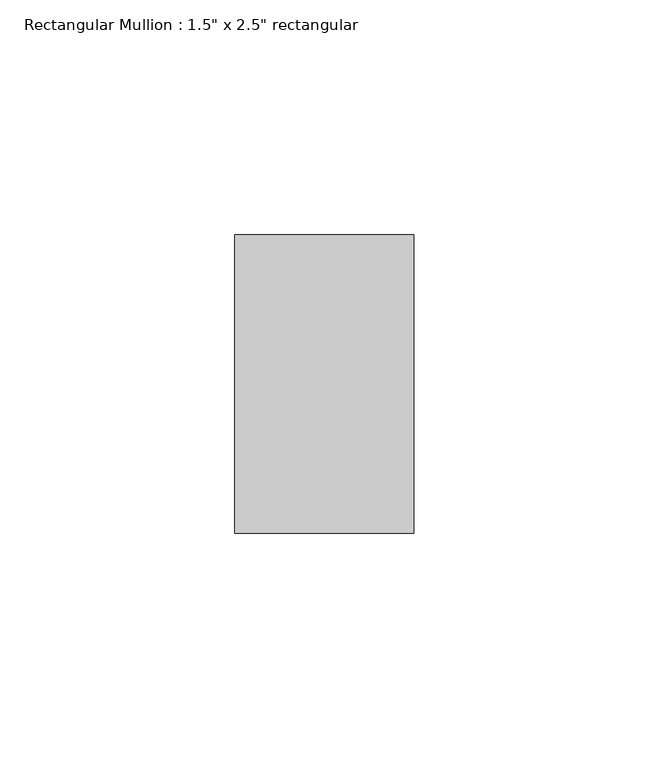
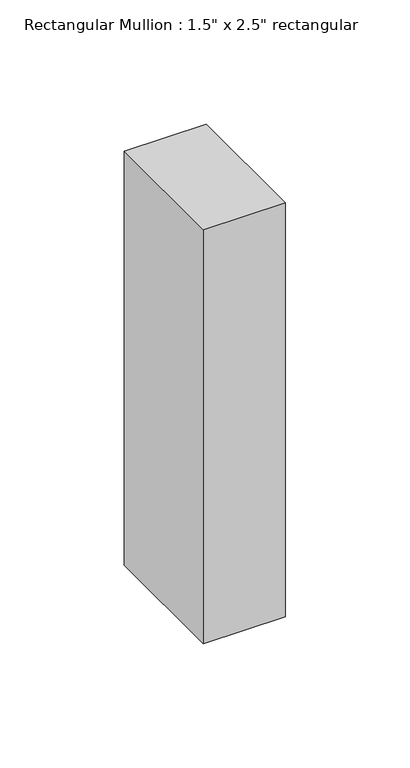
"""IFC4 building model written with IfcOpenShell, lengths in millimetres: member geometry."""

from ifc_helpers import new_model, si_unit, frame, origin, place, context, project, spatial, polyline, outline, extrude, source, transform, mapped, element, save


def member_ff422208(model_context):
    return source(origin(), model_context, "Body", "SweptSolid", [
        extrude(outline(polyline([(0.0, 31.75), (0.0, -31.75), (-38.1, -31.75), (-38.1, 31.75), (0.0, 31.75)])), frame((0.0, 0.0, -203.2), z_axis=(0.0, 0.0, 1.0), x_axis=(1.0, 0.0, 0.0)), (0.0, 0.0, 1.0), 203.2),
    ])


if __name__ == "__main__":
    model = new_model("IFC4")
    model_context = context("Model", 3, world=origin())
    ifc_project = project(units=[si_unit("LENGTHUNIT", "METRE", prefix="MILLI")], contexts=[model_context])
    site = spatial("IfcSite", under=ifc_project)
    building = spatial("IfcBuilding", under=site)
    placement = place(None, origin())
    member_shape = member_ff422208(model_context)
    element("IfcMember", 1, ObjectType="Rectangular Mullion : 1.5\" x 2.5\" rectangular", at=placement, inside=building, context=model_context, shape_type="MappedRepresentation", body=[
        mapped(member_shape, transform((0.0, 0.0, 0.0), x_axis=(1.0, 0.0, 0.0), y_axis=(0.0, 1.0, 0.0), z_axis=(0.0, 0.0, 1.0))),
    ])
    save(model, "model.ifc")

# Revit data of these elements
# Type "Rectangular Mullion : 1.5\" x 2.5\" rectangular"
#   built-in parameter 1007304 = 0.208333 (stored number, unit not read)
#   built-in parameter 1007301 = 0.0625 (stored number, unit not read)
#   built-in parameter 1007300 = 0.0625 (stored number, unit not read)
# Element 1 (IfcMember, "Rectangular Mullion : 1.5\" x 2.5\" rectangular")
#   Materials on its faces: "Aluminum"
# Materials
#   "Aluminum": class "Metal", colour RGB 247 247 247, transparency 0, Description = "Aluminum 6061", Cost = 0
